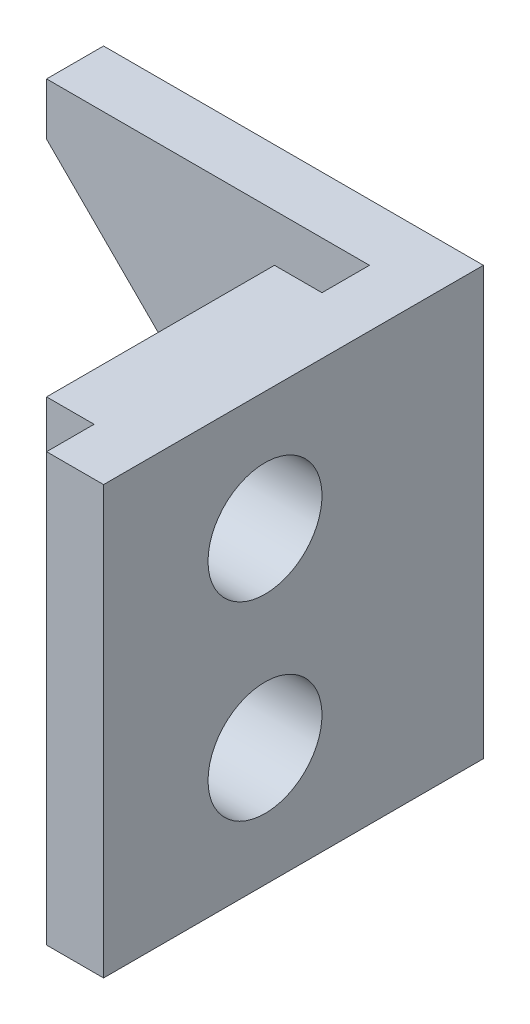
ISO-10303-21;
HEADER;
FILE_DESCRIPTION(('STEP AP214'),'2;1');
FILE_NAME('part.step','',(''),(''),'','','');
FILE_SCHEMA(('AUTOMOTIVE_DESIGN { 1 0 10303 214 1 1 1 1 }'));
ENDSEC;
DATA;
#1=APPLICATION_CONTEXT('core data for automotive mechanical design processes');
#2=APPLICATION_PROTOCOL_DEFINITION('international standard','automotive_design',2000,#1);
#3=PRODUCT_CONTEXT('',#1,'mechanical');
#4=PRODUCT('Part','Part','',(#3));
#5=PRODUCT_RELATED_PRODUCT_CATEGORY('part','',(#4));
#6=PRODUCT_DEFINITION_FORMATION('','',#4);
#7=PRODUCT_DEFINITION_CONTEXT('part definition',#1,'design');
#8=PRODUCT_DEFINITION('design','',#6,#7);
#9=PRODUCT_DEFINITION_SHAPE('','',#8);
#10=(LENGTH_UNIT() NAMED_UNIT(*) SI_UNIT(.MILLI.,.METRE.));
#11=(NAMED_UNIT(*) PLANE_ANGLE_UNIT() SI_UNIT($,.RADIAN.));
#12=(NAMED_UNIT(*) SI_UNIT($,.STERADIAN.) SOLID_ANGLE_UNIT());
#13=UNCERTAINTY_MEASURE_WITH_UNIT(LENGTH_MEASURE(1.E-05),#10,'distance_accuracy_value','');
#14=(GEOMETRIC_REPRESENTATION_CONTEXT(3) GLOBAL_UNCERTAINTY_ASSIGNED_CONTEXT((#13)) GLOBAL_UNIT_ASSIGNED_CONTEXT((#10,
#11,#12)) REPRESENTATION_CONTEXT('',''));
#15=CARTESIAN_POINT('',(0.,0.,0.));
#16=DIRECTION('',(0.,0.,1.));
#17=DIRECTION('',(1.,0.,0.));
#18=AXIS2_PLACEMENT_3D('',#15,#16,#17);
#19=CARTESIAN_POINT('',(0.,0.,6.));
#20=DIRECTION('',(0.,0.,1.));
#21=DIRECTION('',(1.,0.,0.));
#22=AXIS2_PLACEMENT_3D('',#19,#20,#21);
#23=PLANE('',#22);
#24=DIRECTION('',(0.,-1.,0.));
#25=VECTOR('',#24,1.);
#26=CARTESIAN_POINT('',(0.,45.,6.));
#27=LINE('',#26,#25);
#28=CARTESIAN_POINT('',(0.,45.,6.));
#29=VERTEX_POINT('',#28);
#30=CARTESIAN_POINT('',(0.,39.5,6.));
#31=VERTEX_POINT('',#30);
#32=EDGE_CURVE('E179',#29,#31,#27,.T.);
#33=ORIENTED_EDGE('',*,*,#32,.T.);
#34=DIRECTION('',(0.707106781186546,-0.707106781186549,0.));
#35=VECTOR('',#34,1.);
#36=CARTESIAN_POINT('',(19.75,19.75,6.));
#37=LINE('',#36,#35);
#38=CARTESIAN_POINT('',(14.5,25.,6.));
#39=VERTEX_POINT('',#38);
#40=EDGE_CURVE('E160',#31,#39,#37,.T.);
#41=ORIENTED_EDGE('',*,*,#40,.T.);
#42=DIRECTION('',(-1.,0.,0.));
#43=VECTOR('',#42,1.);
#44=CARTESIAN_POINT('',(0.,25.,6.));
#45=LINE('',#44,#43);
#46=CARTESIAN_POINT('',(17.,25.,6.));
#47=VERTEX_POINT('',#46);
#48=EDGE_CURVE('E177',#47,#39,#45,.T.);
#49=ORIENTED_EDGE('',*,*,#48,.F.);
#50=DIRECTION('',(0.,1.,0.));
#51=VECTOR('',#50,1.);
#52=CARTESIAN_POINT('',(17.,0.,6.));
#53=LINE('',#52,#51);
#54=CARTESIAN_POINT('',(17.,20.,6.));
#55=VERTEX_POINT('',#54);
#56=EDGE_CURVE('E232',#55,#47,#53,.T.);
#57=ORIENTED_EDGE('',*,*,#56,.F.);
#58=DIRECTION('',(-1.,0.,0.));
#59=VECTOR('',#58,1.);
#60=CARTESIAN_POINT('',(0.,20.,6.));
#61=LINE('',#60,#59);
#62=CARTESIAN_POINT('',(14.5,20.,6.));
#63=VERTEX_POINT('',#62);
#64=EDGE_CURVE('E320',#55,#63,#61,.T.);
#65=ORIENTED_EDGE('',*,*,#64,.T.);
#66=DIRECTION('',(0.707106781186546,0.707106781186549,0.));
#67=VECTOR('',#66,1.);
#68=CARTESIAN_POINT('',(-2.74999999999997,2.74999999999996,6.));
#69=LINE('',#68,#67);
#70=CARTESIAN_POINT('',(0.,5.49999999999994,6.));
#71=VERTEX_POINT('',#70);
#72=EDGE_CURVE('E169',#71,#63,#69,.T.);
#73=ORIENTED_EDGE('',*,*,#72,.F.);
#74=CARTESIAN_POINT('',(0.,0.,6.));
#75=VERTEX_POINT('',#74);
#76=EDGE_CURVE('E190',#71,#75,#27,.T.);
#77=ORIENTED_EDGE('',*,*,#76,.T.);
#78=DIRECTION('',(1.,0.,0.));
#79=VECTOR('',#78,1.);
#80=CARTESIAN_POINT('',(0.,0.,6.));
#81=LINE('',#80,#79);
#82=CARTESIAN_POINT('',(34.,0.,6.));
#83=VERTEX_POINT('',#82);
#84=EDGE_CURVE('E186',#75,#83,#81,.T.);
#85=ORIENTED_EDGE('',*,*,#84,.T.);
#86=DIRECTION('',(0.,1.,0.));
#87=VECTOR('',#86,1.);
#88=CARTESIAN_POINT('',(34.,0.,6.));
#89=LINE('',#88,#87);
#90=CARTESIAN_POINT('',(34.,45.,6.));
#91=VERTEX_POINT('',#90);
#92=EDGE_CURVE('E268',#83,#91,#89,.T.);
#93=ORIENTED_EDGE('',*,*,#92,.T.);
#94=DIRECTION('',(-1.,0.,0.));
#95=VECTOR('',#94,1.);
#96=CARTESIAN_POINT('',(40.,45.,6.));
#97=LINE('',#96,#95);
#98=EDGE_CURVE('E184',#91,#29,#97,.T.);
#99=ORIENTED_EDGE('',*,*,#98,.T.);
#100=EDGE_LOOP('',(#33,#41,#49,#57,#65,#73,#77,#85,#93,#99));
#101=FACE_BOUND('',#100,.T.);
#102=ADVANCED_FACE('F44',(#101),#23,.T.);
#103=CARTESIAN_POINT('',(0.,45.,6.));
#104=DIRECTION('',(1.,0.,0.));
#105=DIRECTION('',(0.,0.,-1.));
#106=AXIS2_PLACEMENT_3D('',#103,#104,#105);
#107=PLANE('',#106);
#108=DIRECTION('',(0.,0.,1.));
#109=VECTOR('',#108,1.);
#110=CARTESIAN_POINT('',(0.,39.5,-39.));
#111=LINE('',#110,#109);
#112=CARTESIAN_POINT('',(0.,39.5,0.));
#113=VERTEX_POINT('',#112);
#114=EDGE_CURVE('E159',#113,#31,#111,.T.);
#115=ORIENTED_EDGE('',*,*,#114,.T.);
#116=ORIENTED_EDGE('',*,*,#32,.F.);
#117=DIRECTION('',(0.,0.,-1.));
#118=VECTOR('',#117,1.);
#119=CARTESIAN_POINT('',(0.,45.,6.));
#120=LINE('',#119,#118);
#121=CARTESIAN_POINT('',(0.,45.,0.));
#122=VERTEX_POINT('',#121);
#123=EDGE_CURVE('E197',#29,#122,#120,.T.);
#124=ORIENTED_EDGE('',*,*,#123,.T.);
#125=DIRECTION('',(0.,-1.,0.));
#126=VECTOR('',#125,1.);
#127=CARTESIAN_POINT('',(0.,45.,0.));
#128=LINE('',#127,#126);
#129=EDGE_CURVE('E180',#122,#113,#128,.T.);
#130=ORIENTED_EDGE('',*,*,#129,.T.);
#131=EDGE_LOOP('',(#115,#116,#124,#130));
#132=FACE_BOUND('',#131,.T.);
#133=ADVANCED_FACE('F173',(#132),#107,.F.);
#134=CARTESIAN_POINT('',(0.,0.,0.));
#135=DIRECTION('',(0.,0.,1.));
#136=DIRECTION('',(1.,0.,0.));
#137=AXIS2_PLACEMENT_3D('',#134,#135,#136);
#138=PLANE('',#137);
#139=DIRECTION('',(0.707106781186546,-0.707106781186549,0.));
#140=VECTOR('',#139,1.);
#141=CARTESIAN_POINT('',(19.75,19.75,0.));
#142=LINE('',#141,#140);
#143=CARTESIAN_POINT('',(14.5,25.,0.));
#144=VERTEX_POINT('',#143);
#145=EDGE_CURVE('E11',#113,#144,#142,.T.);
#146=ORIENTED_EDGE('',*,*,#145,.F.);
#147=ORIENTED_EDGE('',*,*,#129,.F.);
#148=DIRECTION('',(-1.,0.,0.));
#149=VECTOR('',#148,1.);
#150=CARTESIAN_POINT('',(40.,45.,0.));
#151=LINE('',#150,#149);
#152=CARTESIAN_POINT('',(40.,45.,0.));
#153=VERTEX_POINT('',#152);
#154=EDGE_CURVE('E194',#153,#122,#151,.T.);
#155=ORIENTED_EDGE('',*,*,#154,.F.);
#156=DIRECTION('',(0.,1.,0.));
#157=VECTOR('',#156,1.);
#158=CARTESIAN_POINT('',(40.,0.,0.));
#159=LINE('',#158,#157);
#160=CARTESIAN_POINT('',(40.,0.,0.));
#161=VERTEX_POINT('',#160);
#162=EDGE_CURVE('E205',#161,#153,#159,.T.);
#163=ORIENTED_EDGE('',*,*,#162,.F.);
#164=DIRECTION('',(1.,0.,0.));
#165=VECTOR('',#164,1.);
#166=CARTESIAN_POINT('',(0.,0.,0.));
#167=LINE('',#166,#165);
#168=CARTESIAN_POINT('',(0.,0.,0.));
#169=VERTEX_POINT('',#168);
#170=EDGE_CURVE('E200',#169,#161,#167,.T.);
#171=ORIENTED_EDGE('',*,*,#170,.F.);
#172=CARTESIAN_POINT('',(0.,5.49999999999994,0.));
#173=VERTEX_POINT('',#172);
#174=EDGE_CURVE('E199',#173,#169,#128,.T.);
#175=ORIENTED_EDGE('',*,*,#174,.F.);
#176=DIRECTION('',(0.707106781186546,0.707106781186549,0.));
#177=VECTOR('',#176,1.);
#178=CARTESIAN_POINT('',(-2.74999999999997,2.74999999999996,0.));
#179=LINE('',#178,#177);
#180=CARTESIAN_POINT('',(14.5,20.,0.));
#181=VERTEX_POINT('',#180);
#182=EDGE_CURVE('E214',#173,#181,#179,.T.);
#183=ORIENTED_EDGE('',*,*,#182,.T.);
#184=DIRECTION('',(-1.,0.,0.));
#185=VECTOR('',#184,1.);
#186=CARTESIAN_POINT('',(0.,20.,0.));
#187=LINE('',#186,#185);
#188=CARTESIAN_POINT('',(17.,20.,0.));
#189=VERTEX_POINT('',#188);
#190=EDGE_CURVE('E217',#189,#181,#187,.T.);
#191=ORIENTED_EDGE('',*,*,#190,.F.);
#192=DIRECTION('',(0.,1.,0.));
#193=VECTOR('',#192,1.);
#194=CARTESIAN_POINT('',(17.,0.,0.));
#195=LINE('',#194,#193);
#196=CARTESIAN_POINT('',(17.,25.,0.));
#197=VERTEX_POINT('',#196);
#198=EDGE_CURVE('E219',#189,#197,#195,.T.);
#199=ORIENTED_EDGE('',*,*,#198,.T.);
#200=DIRECTION('',(-1.,0.,0.));
#201=VECTOR('',#200,1.);
#202=CARTESIAN_POINT('',(0.,25.,0.));
#203=LINE('',#202,#201);
#204=EDGE_CURVE('E52',#197,#144,#203,.T.);
#205=ORIENTED_EDGE('',*,*,#204,.T.);
#206=EDGE_LOOP('',(#146,#147,#155,#163,#171,#175,#183,#191,#199,#205));
#207=FACE_BOUND('',#206,.T.);
#208=ADVANCED_FACE('F221',(#207),#138,.F.);
#209=CARTESIAN_POINT('',(34.,0.,0.));
#210=DIRECTION('',(1.,0.,0.));
#211=DIRECTION('',(0.,0.,-1.));
#212=AXIS2_PLACEMENT_3D('',#209,#210,#211);
#213=PLANE('',#212);
#214=DIRECTION('',(0.,0.,-1.));
#215=VECTOR('',#214,1.);
#216=CARTESIAN_POINT('',(34.,0.,40.));
#217=LINE('',#216,#215);
#218=CARTESIAN_POINT('',(34.,0.,11.));
#219=VERTEX_POINT('',#218);
#220=EDGE_CURVE('E280',#219,#83,#217,.T.);
#221=ORIENTED_EDGE('',*,*,#220,.F.);
#222=DIRECTION('',(0.,-1.,0.));
#223=VECTOR('',#222,1.);
#224=CARTESIAN_POINT('',(34.,45.,11.));
#225=LINE('',#224,#223);
#226=CARTESIAN_POINT('',(34.,45.,11.));
#227=VERTEX_POINT('',#226);
#228=EDGE_CURVE('E259',#227,#219,#225,.T.);
#229=ORIENTED_EDGE('',*,*,#228,.F.);
#230=DIRECTION('',(0.,0.,1.));
#231=VECTOR('',#230,1.);
#232=CARTESIAN_POINT('',(34.,45.,6.));
#233=LINE('',#232,#231);
#234=EDGE_CURVE('E271',#91,#227,#233,.T.);
#235=ORIENTED_EDGE('',*,*,#234,.F.);
#236=ORIENTED_EDGE('',*,*,#92,.F.);
#237=EDGE_LOOP('',(#221,#229,#235,#236));
#238=FACE_BOUND('',#237,.T.);
#239=ADVANCED_FACE('F308',(#238),#213,.F.);
#240=ORIENTED_EDGE('',*,*,#76,.F.);
#241=DIRECTION('',(0.,0.,1.));
#242=VECTOR('',#241,1.);
#243=CARTESIAN_POINT('',(0.,5.49999999999994,-39.));
#244=LINE('',#243,#242);
#245=EDGE_CURVE('E178',#173,#71,#244,.T.);
#246=ORIENTED_EDGE('',*,*,#245,.F.);
#247=ORIENTED_EDGE('',*,*,#174,.T.);
#248=DIRECTION('',(0.,0.,-1.));
#249=VECTOR('',#248,1.);
#250=CARTESIAN_POINT('',(0.,0.,6.));
#251=LINE('',#250,#249);
#252=EDGE_CURVE('E215',#75,#169,#251,.T.);
#253=ORIENTED_EDGE('',*,*,#252,.F.);
#254=EDGE_LOOP('',(#240,#246,#247,#253));
#255=FACE_BOUND('',#254,.T.);
#256=ADVANCED_FACE('F50',(#255),#107,.F.);
#257=CARTESIAN_POINT('',(0.,0.,6.));
#258=DIRECTION('',(0.,1.,0.));
#259=DIRECTION('',(0.,0.,1.));
#260=AXIS2_PLACEMENT_3D('',#257,#258,#259);
#261=PLANE('',#260);
#262=ORIENTED_EDGE('',*,*,#170,.T.);
#263=DIRECTION('',(0.,0.,-1.));
#264=VECTOR('',#263,1.);
#265=CARTESIAN_POINT('',(40.,0.,6.));
#266=LINE('',#265,#264);
#267=CARTESIAN_POINT('',(40.,0.,40.));
#268=VERTEX_POINT('',#267);
#269=EDGE_CURVE('E207',#268,#161,#266,.T.);
#270=ORIENTED_EDGE('',*,*,#269,.F.);
#271=DIRECTION('',(1.,0.,0.));
#272=VECTOR('',#271,1.);
#273=CARTESIAN_POINT('',(34.,0.,40.));
#274=LINE('',#273,#272);
#275=CARTESIAN_POINT('',(34.,0.,40.));
#276=VERTEX_POINT('',#275);
#277=EDGE_CURVE('E285',#276,#268,#274,.T.);
#278=ORIENTED_EDGE('',*,*,#277,.F.);
#279=CARTESIAN_POINT('',(34.,0.,35.));
#280=VERTEX_POINT('',#279);
#281=EDGE_CURVE('E279',#276,#280,#217,.T.);
#282=ORIENTED_EDGE('',*,*,#281,.T.);
#283=DIRECTION('',(-1.,0.,0.));
#284=VECTOR('',#283,1.);
#285=CARTESIAN_POINT('',(34.,0.,35.));
#286=LINE('',#285,#284);
#287=CARTESIAN_POINT('',(29.,0.,35.));
#288=VERTEX_POINT('',#287);
#289=EDGE_CURVE('E236',#280,#288,#286,.T.);
#290=ORIENTED_EDGE('',*,*,#289,.T.);
#291=DIRECTION('',(0.,0.,-1.));
#292=VECTOR('',#291,1.);
#293=CARTESIAN_POINT('',(29.,0.,35.));
#294=LINE('',#293,#292);
#295=CARTESIAN_POINT('',(29.,0.,11.));
#296=VERTEX_POINT('',#295);
#297=EDGE_CURVE('E258',#288,#296,#294,.T.);
#298=ORIENTED_EDGE('',*,*,#297,.T.);
#299=DIRECTION('',(1.,0.,0.));
#300=VECTOR('',#299,1.);
#301=CARTESIAN_POINT('',(29.,0.,11.));
#302=LINE('',#301,#300);
#303=EDGE_CURVE('E70',#296,#219,#302,.T.);
#304=ORIENTED_EDGE('',*,*,#303,.T.);
#305=ORIENTED_EDGE('',*,*,#220,.T.);
#306=ORIENTED_EDGE('',*,*,#84,.F.);
#307=ORIENTED_EDGE('',*,*,#252,.T.);
#308=EDGE_LOOP('',(#262,#270,#278,#282,#290,#298,#304,#305,#306,#307));
#309=FACE_BOUND('',#308,.T.);
#310=ADVANCED_FACE('F313',(#309),#261,.F.);
#311=CARTESIAN_POINT('',(40.,0.,6.));
#312=DIRECTION('',(-1.,0.,0.));
#313=DIRECTION('',(0.,0.,1.));
#314=AXIS2_PLACEMENT_3D('',#311,#312,#313);
#315=PLANE('',#314);
#316=CARTESIAN_POINT('',(40.,32.5,23.));
#317=DIRECTION('',(-1.,0.,0.));
#318=DIRECTION('',(0.,0.,1.));
#319=AXIS2_PLACEMENT_3D('',#316,#317,#318);
#320=CIRCLE('',#319,6.);
#321=CARTESIAN_POINT('',(40.,32.5,29.));
#322=VERTEX_POINT('',#321);
#323=EDGE_CURVE('E166',#322,#322,#320,.T.);
#324=ORIENTED_EDGE('',*,*,#323,.T.);
#325=EDGE_LOOP('',(#324));
#326=FACE_BOUND('',#325,.T.);
#327=CARTESIAN_POINT('',(40.,12.5,23.));
#328=DIRECTION('',(-1.,0.,0.));
#329=DIRECTION('',(0.,0.,1.));
#330=AXIS2_PLACEMENT_3D('',#327,#328,#329);
#331=CIRCLE('',#330,6.);
#332=CARTESIAN_POINT('',(40.,12.5,29.));
#333=VERTEX_POINT('',#332);
#334=EDGE_CURVE('E322',#333,#333,#331,.T.);
#335=ORIENTED_EDGE('',*,*,#334,.T.);
#336=EDGE_LOOP('',(#335));
#337=FACE_BOUND('',#336,.T.);
#338=ORIENTED_EDGE('',*,*,#162,.T.);
#339=DIRECTION('',(0.,0.,-1.));
#340=VECTOR('',#339,1.);
#341=CARTESIAN_POINT('',(40.,45.,6.));
#342=LINE('',#341,#340);
#343=CARTESIAN_POINT('',(40.,45.,40.));
#344=VERTEX_POINT('',#343);
#345=EDGE_CURVE('E206',#344,#153,#342,.T.);
#346=ORIENTED_EDGE('',*,*,#345,.F.);
#347=DIRECTION('',(0.,-1.,0.));
#348=VECTOR('',#347,1.);
#349=CARTESIAN_POINT('',(40.,45.,40.));
#350=LINE('',#349,#348);
#351=EDGE_CURVE('E261',#344,#268,#350,.T.);
#352=ORIENTED_EDGE('',*,*,#351,.T.);
#353=ORIENTED_EDGE('',*,*,#269,.T.);
#354=EDGE_LOOP('',(#338,#346,#352,#353));
#355=FACE_BOUND('',#354,.T.);
#356=ADVANCED_FACE('F296',(#326,#337,#355),#315,.F.);
#357=CARTESIAN_POINT('',(40.,45.,6.));
#358=DIRECTION('',(0.,-1.,0.));
#359=DIRECTION('',(0.,0.,-1.));
#360=AXIS2_PLACEMENT_3D('',#357,#358,#359);
#361=PLANE('',#360);
#362=ORIENTED_EDGE('',*,*,#154,.T.);
#363=ORIENTED_EDGE('',*,*,#123,.F.);
#364=ORIENTED_EDGE('',*,*,#98,.F.);
#365=ORIENTED_EDGE('',*,*,#234,.T.);
#366=DIRECTION('',(1.,0.,0.));
#367=VECTOR('',#366,1.);
#368=CARTESIAN_POINT('',(29.,45.,11.));
#369=LINE('',#368,#367);
#370=CARTESIAN_POINT('',(29.,45.,11.));
#371=VERTEX_POINT('',#370);
#372=EDGE_CURVE('E253',#371,#227,#369,.T.);
#373=ORIENTED_EDGE('',*,*,#372,.F.);
#374=DIRECTION('',(0.,0.,-1.));
#375=VECTOR('',#374,1.);
#376=CARTESIAN_POINT('',(29.,45.,35.));
#377=LINE('',#376,#375);
#378=CARTESIAN_POINT('',(29.,45.,35.));
#379=VERTEX_POINT('',#378);
#380=EDGE_CURVE('E250',#379,#371,#377,.T.);
#381=ORIENTED_EDGE('',*,*,#380,.F.);
#382=DIRECTION('',(-1.,0.,0.));
#383=VECTOR('',#382,1.);
#384=CARTESIAN_POINT('',(34.,45.,35.));
#385=LINE('',#384,#383);
#386=CARTESIAN_POINT('',(34.,45.,35.));
#387=VERTEX_POINT('',#386);
#388=EDGE_CURVE('E244',#387,#379,#385,.T.);
#389=ORIENTED_EDGE('',*,*,#388,.F.);
#390=CARTESIAN_POINT('',(34.,45.,40.));
#391=VERTEX_POINT('',#390);
#392=EDGE_CURVE('E269',#387,#391,#233,.T.);
#393=ORIENTED_EDGE('',*,*,#392,.T.);
#394=DIRECTION('',(1.,0.,0.));
#395=VECTOR('',#394,1.);
#396=CARTESIAN_POINT('',(34.,45.,40.));
#397=LINE('',#396,#395);
#398=EDGE_CURVE('E195',#391,#344,#397,.T.);
#399=ORIENTED_EDGE('',*,*,#398,.T.);
#400=ORIENTED_EDGE('',*,*,#345,.T.);
#401=EDGE_LOOP('',(#362,#363,#364,#365,#373,#381,#389,#393,#399,#400));
#402=FACE_BOUND('',#401,.T.);
#403=ADVANCED_FACE('F288',(#402),#361,.F.);
#404=CARTESIAN_POINT('',(34.,45.,40.));
#405=DIRECTION('',(0.,0.,1.));
#406=DIRECTION('',(1.,0.,0.));
#407=AXIS2_PLACEMENT_3D('',#404,#405,#406);
#408=PLANE('',#407);
#409=ORIENTED_EDGE('',*,*,#351,.F.);
#410=ORIENTED_EDGE('',*,*,#398,.F.);
#411=DIRECTION('',(0.,-1.,0.));
#412=VECTOR('',#411,1.);
#413=CARTESIAN_POINT('',(34.,45.,40.));
#414=LINE('',#413,#412);
#415=EDGE_CURVE('E273',#391,#276,#414,.T.);
#416=ORIENTED_EDGE('',*,*,#415,.T.);
#417=ORIENTED_EDGE('',*,*,#277,.T.);
#418=EDGE_LOOP('',(#409,#410,#416,#417));
#419=FACE_BOUND('',#418,.T.);
#420=ADVANCED_FACE('F294',(#419),#408,.T.);
#421=ORIENTED_EDGE('',*,*,#392,.F.);
#422=DIRECTION('',(0.,-1.,0.));
#423=VECTOR('',#422,1.);
#424=CARTESIAN_POINT('',(34.,45.,35.));
#425=LINE('',#424,#423);
#426=EDGE_CURVE('E251',#387,#280,#425,.T.);
#427=ORIENTED_EDGE('',*,*,#426,.T.);
#428=ORIENTED_EDGE('',*,*,#281,.F.);
#429=ORIENTED_EDGE('',*,*,#415,.F.);
#430=EDGE_LOOP('',(#421,#427,#428,#429));
#431=FACE_BOUND('',#430,.T.);
#432=ADVANCED_FACE('F349',(#431),#213,.F.);
#433=CARTESIAN_POINT('',(29.,45.,11.));
#434=DIRECTION('',(0.,0.,-1.));
#435=DIRECTION('',(-1.,0.,0.));
#436=AXIS2_PLACEMENT_3D('',#433,#434,#435);
#437=PLANE('',#436);
#438=ORIENTED_EDGE('',*,*,#303,.F.);
#439=DIRECTION('',(0.,-1.,0.));
#440=VECTOR('',#439,1.);
#441=CARTESIAN_POINT('',(29.,45.,11.));
#442=LINE('',#441,#440);
#443=EDGE_CURVE('E265',#371,#296,#442,.T.);
#444=ORIENTED_EDGE('',*,*,#443,.F.);
#445=ORIENTED_EDGE('',*,*,#372,.T.);
#446=ORIENTED_EDGE('',*,*,#228,.T.);
#447=EDGE_LOOP('',(#438,#444,#445,#446));
#448=FACE_BOUND('',#447,.T.);
#449=ADVANCED_FACE('F344',(#448),#437,.T.);
#450=CARTESIAN_POINT('',(29.,45.,35.));
#451=DIRECTION('',(-1.,0.,0.));
#452=DIRECTION('',(0.,0.,1.));
#453=AXIS2_PLACEMENT_3D('',#450,#451,#452);
#454=PLANE('',#453);
#455=CARTESIAN_POINT('',(29.,32.5,23.));
#456=DIRECTION('',(-1.,0.,0.));
#457=DIRECTION('',(0.,0.,1.));
#458=AXIS2_PLACEMENT_3D('',#455,#456,#457);
#459=CIRCLE('',#458,6.);
#460=CARTESIAN_POINT('',(29.,32.5,29.));
#461=VERTEX_POINT('',#460);
#462=EDGE_CURVE('E330',#461,#461,#459,.T.);
#463=ORIENTED_EDGE('',*,*,#462,.F.);
#464=EDGE_LOOP('',(#463));
#465=FACE_BOUND('',#464,.T.);
#466=CARTESIAN_POINT('',(29.,12.5,23.));
#467=DIRECTION('',(-1.,0.,0.));
#468=DIRECTION('',(0.,0.,1.));
#469=AXIS2_PLACEMENT_3D('',#466,#467,#468);
#470=CIRCLE('',#469,6.);
#471=CARTESIAN_POINT('',(29.,12.5,29.));
#472=VERTEX_POINT('',#471);
#473=EDGE_CURVE('E327',#472,#472,#470,.T.);
#474=ORIENTED_EDGE('',*,*,#473,.F.);
#475=EDGE_LOOP('',(#474));
#476=FACE_BOUND('',#475,.T.);
#477=ORIENTED_EDGE('',*,*,#297,.F.);
#478=DIRECTION('',(0.,-1.,0.));
#479=VECTOR('',#478,1.);
#480=CARTESIAN_POINT('',(29.,45.,35.));
#481=LINE('',#480,#479);
#482=EDGE_CURVE('E262',#379,#288,#481,.T.);
#483=ORIENTED_EDGE('',*,*,#482,.F.);
#484=ORIENTED_EDGE('',*,*,#380,.T.);
#485=ORIENTED_EDGE('',*,*,#443,.T.);
#486=EDGE_LOOP('',(#477,#483,#484,#485));
#487=FACE_BOUND('',#486,.T.);
#488=ADVANCED_FACE('F340',(#465,#476,#487),#454,.T.);
#489=CARTESIAN_POINT('',(34.,45.,35.));
#490=DIRECTION('',(0.,0.,1.));
#491=DIRECTION('',(1.,0.,0.));
#492=AXIS2_PLACEMENT_3D('',#489,#490,#491);
#493=PLANE('',#492);
#494=ORIENTED_EDGE('',*,*,#289,.F.);
#495=ORIENTED_EDGE('',*,*,#426,.F.);
#496=ORIENTED_EDGE('',*,*,#388,.T.);
#497=ORIENTED_EDGE('',*,*,#482,.T.);
#498=EDGE_LOOP('',(#494,#495,#496,#497));
#499=FACE_BOUND('',#498,.T.);
#500=ADVANCED_FACE('F339',(#499),#493,.T.);
#501=CARTESIAN_POINT('',(19.75,19.75,-39.));
#502=DIRECTION('',(-0.707106781186549,-0.707106781186546,0.));
#503=DIRECTION('',(0.707106781186546,-0.707106781186549,0.));
#504=AXIS2_PLACEMENT_3D('',#501,#502,#503);
#505=PLANE('',#504);
#506=ORIENTED_EDGE('',*,*,#145,.T.);
#507=DIRECTION('',(0.,0.,1.));
#508=VECTOR('',#507,1.);
#509=CARTESIAN_POINT('',(14.5,25.,-39.));
#510=LINE('',#509,#508);
#511=EDGE_CURVE('E162',#144,#39,#510,.T.);
#512=ORIENTED_EDGE('',*,*,#511,.T.);
#513=ORIENTED_EDGE('',*,*,#40,.F.);
#514=ORIENTED_EDGE('',*,*,#114,.F.);
#515=EDGE_LOOP('',(#506,#512,#513,#514));
#516=FACE_BOUND('',#515,.T.);
#517=ADVANCED_FACE('F157',(#516),#505,.T.);
#518=CARTESIAN_POINT('',(0.,25.,-39.));
#519=DIRECTION('',(0.,1.,0.));
#520=DIRECTION('',(0.,0.,1.));
#521=AXIS2_PLACEMENT_3D('',#518,#519,#520);
#522=PLANE('',#521);
#523=DIRECTION('',(0.,0.,1.));
#524=VECTOR('',#523,1.);
#525=CARTESIAN_POINT('',(17.,25.,-39.));
#526=LINE('',#525,#524);
#527=EDGE_CURVE('E228',#197,#47,#526,.T.);
#528=ORIENTED_EDGE('',*,*,#527,.T.);
#529=ORIENTED_EDGE('',*,*,#48,.T.);
#530=ORIENTED_EDGE('',*,*,#511,.F.);
#531=ORIENTED_EDGE('',*,*,#204,.F.);
#532=EDGE_LOOP('',(#528,#529,#530,#531));
#533=FACE_BOUND('',#532,.T.);
#534=ADVANCED_FACE('F227',(#533),#522,.F.);
#535=CARTESIAN_POINT('',(17.,0.,-39.));
#536=DIRECTION('',(1.,0.,0.));
#537=DIRECTION('',(0.,0.,-1.));
#538=AXIS2_PLACEMENT_3D('',#535,#536,#537);
#539=PLANE('',#538);
#540=DIRECTION('',(0.,0.,1.));
#541=VECTOR('',#540,1.);
#542=CARTESIAN_POINT('',(17.,20.,-39.));
#543=LINE('',#542,#541);
#544=EDGE_CURVE('E237',#189,#55,#543,.T.);
#545=ORIENTED_EDGE('',*,*,#544,.T.);
#546=ORIENTED_EDGE('',*,*,#56,.T.);
#547=ORIENTED_EDGE('',*,*,#527,.F.);
#548=ORIENTED_EDGE('',*,*,#198,.F.);
#549=EDGE_LOOP('',(#545,#546,#547,#548));
#550=FACE_BOUND('',#549,.T.);
#551=ADVANCED_FACE('F231',(#550),#539,.F.);
#552=CARTESIAN_POINT('',(0.,20.,-39.));
#553=DIRECTION('',(0.,1.,0.));
#554=DIRECTION('',(0.,0.,1.));
#555=AXIS2_PLACEMENT_3D('',#552,#553,#554);
#556=PLANE('',#555);
#557=ORIENTED_EDGE('',*,*,#190,.T.);
#558=DIRECTION('',(0.,0.,1.));
#559=VECTOR('',#558,1.);
#560=CARTESIAN_POINT('',(14.5,20.,-39.));
#561=LINE('',#560,#559);
#562=EDGE_CURVE('E58',#181,#63,#561,.T.);
#563=ORIENTED_EDGE('',*,*,#562,.T.);
#564=ORIENTED_EDGE('',*,*,#64,.F.);
#565=ORIENTED_EDGE('',*,*,#544,.F.);
#566=EDGE_LOOP('',(#557,#563,#564,#565));
#567=FACE_BOUND('',#566,.T.);
#568=ADVANCED_FACE('F412',(#567),#556,.T.);
#569=CARTESIAN_POINT('',(-2.74999999999997,2.74999999999996,-39.));
#570=DIRECTION('',(0.707106781186549,-0.707106781186546,0.));
#571=DIRECTION('',(0.707106781186546,0.707106781186549,0.));
#572=AXIS2_PLACEMENT_3D('',#569,#570,#571);
#573=PLANE('',#572);
#574=ORIENTED_EDGE('',*,*,#245,.T.);
#575=ORIENTED_EDGE('',*,*,#72,.T.);
#576=ORIENTED_EDGE('',*,*,#562,.F.);
#577=ORIENTED_EDGE('',*,*,#182,.F.);
#578=EDGE_LOOP('',(#574,#575,#576,#577));
#579=FACE_BOUND('',#578,.T.);
#580=ADVANCED_FACE('F314',(#579),#573,.F.);
#581=CARTESIAN_POINT('',(74.,12.5,23.));
#582=DIRECTION('',(-1.,0.,0.));
#583=DIRECTION('',(0.,0.,1.));
#584=AXIS2_PLACEMENT_3D('',#581,#582,#583);
#585=CYLINDRICAL_SURFACE('',#584,6.);
#586=CARTESIAN_POINT('',(29.,12.5,29.));
#587=CARTESIAN_POINT('',(29.1145833333333,12.5,29.));
#588=CARTESIAN_POINT('',(29.2291666666667,12.5,29.));
#589=CARTESIAN_POINT('',(29.4583333333333,12.5,29.));
#590=CARTESIAN_POINT('',(29.5729166666667,12.5,29.));
#591=CARTESIAN_POINT('',(29.8020833333333,12.5,29.));
#592=CARTESIAN_POINT('',(29.9166666666667,12.5,29.));
#593=CARTESIAN_POINT('',(30.1458333333333,12.5,29.));
#594=CARTESIAN_POINT('',(30.2604166666667,12.5,29.));
#595=CARTESIAN_POINT('',(30.4895833333333,12.5,29.));
#596=CARTESIAN_POINT('',(30.6041666666667,12.5,29.));
#597=CARTESIAN_POINT('',(30.8333333333333,12.5,29.));
#598=CARTESIAN_POINT('',(30.9479166666667,12.5,29.));
#599=CARTESIAN_POINT('',(31.1770833333333,12.5,29.));
#600=CARTESIAN_POINT('',(31.2916666666667,12.5,29.));
#601=CARTESIAN_POINT('',(31.5208333333333,12.5,29.));
#602=CARTESIAN_POINT('',(31.6354166666667,12.5,29.));
#603=CARTESIAN_POINT('',(31.8645833333333,12.5,29.));
#604=CARTESIAN_POINT('',(31.9791666666667,12.5,29.));
#605=CARTESIAN_POINT('',(32.2083333333333,12.5,29.));
#606=CARTESIAN_POINT('',(32.3229166666667,12.5,29.));
#607=CARTESIAN_POINT('',(32.5520833333333,12.5,29.));
#608=CARTESIAN_POINT('',(32.6666666666667,12.5,29.));
#609=CARTESIAN_POINT('',(32.8958333333333,12.5,29.));
#610=CARTESIAN_POINT('',(33.0104166666667,12.5,29.));
#611=CARTESIAN_POINT('',(33.2395833333333,12.5,29.));
#612=CARTESIAN_POINT('',(33.3541666666667,12.5,29.));
#613=CARTESIAN_POINT('',(33.5833333333333,12.5,29.));
#614=CARTESIAN_POINT('',(33.6979166666667,12.5,29.));
#615=CARTESIAN_POINT('',(33.9270833333333,12.5,29.));
#616=CARTESIAN_POINT('',(34.0416666666667,12.5,29.));
#617=CARTESIAN_POINT('',(34.2708333333333,12.5,29.));
#618=CARTESIAN_POINT('',(34.3854166666667,12.5,29.));
#619=CARTESIAN_POINT('',(34.6145833333333,12.5,29.));
#620=CARTESIAN_POINT('',(34.7291666666667,12.5,29.));
#621=CARTESIAN_POINT('',(34.9583333333333,12.5,29.));
#622=CARTESIAN_POINT('',(35.0729166666667,12.5,29.));
#623=CARTESIAN_POINT('',(35.3020833333333,12.5,29.));
#624=CARTESIAN_POINT('',(35.4166666666667,12.5,29.));
#625=CARTESIAN_POINT('',(35.6458333333333,12.5,29.));
#626=CARTESIAN_POINT('',(35.7604166666667,12.5,29.));
#627=CARTESIAN_POINT('',(35.9895833333333,12.5,29.));
#628=CARTESIAN_POINT('',(36.1041666666667,12.5,29.));
#629=CARTESIAN_POINT('',(36.3333333333333,12.5,29.));
#630=CARTESIAN_POINT('',(36.4479166666667,12.5,29.));
#631=CARTESIAN_POINT('',(36.6770833333333,12.5,29.));
#632=CARTESIAN_POINT('',(36.7916666666667,12.5,29.));
#633=CARTESIAN_POINT('',(37.0208333333333,12.5,29.));
#634=CARTESIAN_POINT('',(37.1354166666667,12.5,29.));
#635=CARTESIAN_POINT('',(37.3645833333333,12.5,29.));
#636=CARTESIAN_POINT('',(37.4791666666667,12.5,29.));
#637=CARTESIAN_POINT('',(37.7083333333333,12.5,29.));
#638=CARTESIAN_POINT('',(37.8229166666667,12.5,29.));
#639=CARTESIAN_POINT('',(38.0520833333333,12.5,29.));
#640=CARTESIAN_POINT('',(38.1666666666667,12.5,29.));
#641=CARTESIAN_POINT('',(38.3958333333333,12.5,29.));
#642=CARTESIAN_POINT('',(38.5104166666667,12.5,29.));
#643=CARTESIAN_POINT('',(38.7395833333333,12.5,29.));
#644=CARTESIAN_POINT('',(38.8541666666667,12.5,29.));
#645=CARTESIAN_POINT('',(39.0833333333333,12.5,29.));
#646=CARTESIAN_POINT('',(39.1979166666667,12.5,29.));
#647=CARTESIAN_POINT('',(39.4270833333333,12.5,29.));
#648=CARTESIAN_POINT('',(39.5416666666667,12.5,29.));
#649=CARTESIAN_POINT('',(39.7708333333333,12.5,29.));
#650=CARTESIAN_POINT('',(39.8854166666667,12.5,29.));
#651=CARTESIAN_POINT('',(40.,12.5,29.));
#652=B_SPLINE_CURVE_WITH_KNOTS('',3,(#586,#587,#588,#589,#590,#591,#592,#593,#594,#595,#596,
#597,#598,#599,#600,#601,#602,#603,#604,#605,#606,#607,#608,#609,#610,#611,#612,#613,#614,#615,
#616,#617,#618,#619,#620,#621,#622,#623,#624,#625,#626,#627,#628,#629,#630,#631,#632,#633,#634,
#635,#636,#637,#638,#639,#640,#641,#642,#643,#644,#645,#646,#647,#648,#649,#650,#651),
.UNSPECIFIED.,.F.,.F.,(4,2,2,2,2,2,2,2,2,2,2,2,2,2,2,2,2,2,2,2,2,2,2,2,2,2,2,2,2,2,2,2,4),(0.,
0.343749999999997,0.687500000000001,1.03125,1.375,1.71875,2.0625,2.40625,2.75,3.09375,3.4375,
3.78125,4.125,4.46875,4.8125,5.15625,5.5,5.84374999999999,6.1875,6.53125,6.875,7.21875,7.5625,
7.90625,8.24999999999999,8.59375,8.9375,9.28125,9.62499999999999,9.96875,10.3125,10.65625,11.),.UNSPECIFIED.);
#653=EDGE_CURVE('BSEAM434',#472,#333,#652,.T.);
#654=ORIENTED_EDGE('',*,*,#473,.T.);
#655=ORIENTED_EDGE('',*,*,#334,.F.);
#656=ORIENTED_EDGE('',*,*,#653,.T.);
#657=ORIENTED_EDGE('',*,*,#653,.F.);
#658=EDGE_LOOP('',(#654,#656,#655,#657));
#659=FACE_BOUND('',#658,.T.);
#660=ADVANCED_FACE('F434',(#659),#585,.F.);
#661=CARTESIAN_POINT('',(74.,32.5,23.));
#662=DIRECTION('',(-1.,0.,0.));
#663=DIRECTION('',(0.,0.,1.));
#664=AXIS2_PLACEMENT_3D('',#661,#662,#663);
#665=CYLINDRICAL_SURFACE('',#664,6.);
#666=CARTESIAN_POINT('',(29.,32.5,29.));
#667=CARTESIAN_POINT('',(29.1145833333333,32.5,29.));
#668=CARTESIAN_POINT('',(29.2291666666667,32.5,29.));
#669=CARTESIAN_POINT('',(29.4583333333333,32.5,29.));
#670=CARTESIAN_POINT('',(29.5729166666667,32.5,29.));
#671=CARTESIAN_POINT('',(29.8020833333333,32.5,29.));
#672=CARTESIAN_POINT('',(29.9166666666667,32.5,29.));
#673=CARTESIAN_POINT('',(30.1458333333333,32.5,29.));
#674=CARTESIAN_POINT('',(30.2604166666667,32.5,29.));
#675=CARTESIAN_POINT('',(30.4895833333333,32.5,29.));
#676=CARTESIAN_POINT('',(30.6041666666667,32.5,29.));
#677=CARTESIAN_POINT('',(30.8333333333333,32.5,29.));
#678=CARTESIAN_POINT('',(30.9479166666667,32.5,29.));
#679=CARTESIAN_POINT('',(31.1770833333333,32.5,29.));
#680=CARTESIAN_POINT('',(31.2916666666667,32.5,29.));
#681=CARTESIAN_POINT('',(31.5208333333333,32.5,29.));
#682=CARTESIAN_POINT('',(31.6354166666667,32.5,29.));
#683=CARTESIAN_POINT('',(31.8645833333333,32.5,29.));
#684=CARTESIAN_POINT('',(31.9791666666667,32.5,29.));
#685=CARTESIAN_POINT('',(32.2083333333333,32.5,29.));
#686=CARTESIAN_POINT('',(32.3229166666667,32.5,29.));
#687=CARTESIAN_POINT('',(32.5520833333333,32.5,29.));
#688=CARTESIAN_POINT('',(32.6666666666667,32.5,29.));
#689=CARTESIAN_POINT('',(32.8958333333333,32.5,29.));
#690=CARTESIAN_POINT('',(33.0104166666667,32.5,29.));
#691=CARTESIAN_POINT('',(33.2395833333333,32.5,29.));
#692=CARTESIAN_POINT('',(33.3541666666667,32.5,29.));
#693=CARTESIAN_POINT('',(33.5833333333333,32.5,29.));
#694=CARTESIAN_POINT('',(33.6979166666667,32.5,29.));
#695=CARTESIAN_POINT('',(33.9270833333333,32.5,29.));
#696=CARTESIAN_POINT('',(34.0416666666667,32.5,29.));
#697=CARTESIAN_POINT('',(34.2708333333333,32.5,29.));
#698=CARTESIAN_POINT('',(34.3854166666667,32.5,29.));
#699=CARTESIAN_POINT('',(34.6145833333333,32.5,29.));
#700=CARTESIAN_POINT('',(34.7291666666667,32.5,29.));
#701=CARTESIAN_POINT('',(34.9583333333333,32.5,29.));
#702=CARTESIAN_POINT('',(35.0729166666667,32.5,29.));
#703=CARTESIAN_POINT('',(35.3020833333333,32.5,29.));
#704=CARTESIAN_POINT('',(35.4166666666667,32.5,29.));
#705=CARTESIAN_POINT('',(35.6458333333333,32.5,29.));
#706=CARTESIAN_POINT('',(35.7604166666667,32.5,29.));
#707=CARTESIAN_POINT('',(35.9895833333333,32.5,29.));
#708=CARTESIAN_POINT('',(36.1041666666667,32.5,29.));
#709=CARTESIAN_POINT('',(36.3333333333333,32.5,29.));
#710=CARTESIAN_POINT('',(36.4479166666667,32.5,29.));
#711=CARTESIAN_POINT('',(36.6770833333333,32.5,29.));
#712=CARTESIAN_POINT('',(36.7916666666667,32.5,29.));
#713=CARTESIAN_POINT('',(37.0208333333333,32.5,29.));
#714=CARTESIAN_POINT('',(37.1354166666667,32.5,29.));
#715=CARTESIAN_POINT('',(37.3645833333333,32.5,29.));
#716=CARTESIAN_POINT('',(37.4791666666667,32.5,29.));
#717=CARTESIAN_POINT('',(37.7083333333333,32.5,29.));
#718=CARTESIAN_POINT('',(37.8229166666667,32.5,29.));
#719=CARTESIAN_POINT('',(38.0520833333333,32.5,29.));
#720=CARTESIAN_POINT('',(38.1666666666667,32.5,29.));
#721=CARTESIAN_POINT('',(38.3958333333333,32.5,29.));
#722=CARTESIAN_POINT('',(38.5104166666667,32.5,29.));
#723=CARTESIAN_POINT('',(38.7395833333333,32.5,29.));
#724=CARTESIAN_POINT('',(38.8541666666667,32.5,29.));
#725=CARTESIAN_POINT('',(39.0833333333333,32.5,29.));
#726=CARTESIAN_POINT('',(39.1979166666667,32.5,29.));
#727=CARTESIAN_POINT('',(39.4270833333333,32.5,29.));
#728=CARTESIAN_POINT('',(39.5416666666667,32.5,29.));
#729=CARTESIAN_POINT('',(39.7708333333333,32.5,29.));
#730=CARTESIAN_POINT('',(39.8854166666667,32.5,29.));
#731=CARTESIAN_POINT('',(40.,32.5,29.));
#732=B_SPLINE_CURVE_WITH_KNOTS('',3,(#666,#667,#668,#669,#670,#671,#672,#673,#674,#675,#676,
#677,#678,#679,#680,#681,#682,#683,#684,#685,#686,#687,#688,#689,#690,#691,#692,#693,#694,#695,
#696,#697,#698,#699,#700,#701,#702,#703,#704,#705,#706,#707,#708,#709,#710,#711,#712,#713,#714,
#715,#716,#717,#718,#719,#720,#721,#722,#723,#724,#725,#726,#727,#728,#729,#730,#731),
.UNSPECIFIED.,.F.,.F.,(4,2,2,2,2,2,2,2,2,2,2,2,2,2,2,2,2,2,2,2,2,2,2,2,2,2,2,2,2,2,2,2,4),(0.,
0.343749999999997,0.687500000000001,1.03125,1.375,1.71875,2.0625,2.40625,2.75,3.09375,3.4375,
3.78125,4.125,4.46875,4.8125,5.15625,5.5,5.84374999999999,6.1875,6.53125,6.875,7.21875,7.5625,
7.90625,8.24999999999999,8.59375,8.9375,9.28125,9.62499999999999,9.96875,10.3125,10.65625,11.),.UNSPECIFIED.);
#733=EDGE_CURVE('BSEAM331',#461,#322,#732,.T.);
#734=ORIENTED_EDGE('',*,*,#462,.T.);
#735=ORIENTED_EDGE('',*,*,#323,.F.);
#736=ORIENTED_EDGE('',*,*,#733,.T.);
#737=ORIENTED_EDGE('',*,*,#733,.F.);
#738=EDGE_LOOP('',(#734,#736,#735,#737));
#739=FACE_BOUND('',#738,.T.);
#740=ADVANCED_FACE('F331',(#739),#665,.F.);
#741=CLOSED_SHELL('',(#102,#133,#208,#239,#256,#310,#356,#403,#420,#432,#449,#488,#500,#517,
#534,#551,#568,#580,#660,#740));
#742=MANIFOLD_SOLID_BREP('B2',#741);
#743=ADVANCED_BREP_SHAPE_REPRESENTATION('',(#18,#742),#14);
#744=SHAPE_DEFINITION_REPRESENTATION(#9,#743);
ENDSEC;
END-ISO-10303-21;
